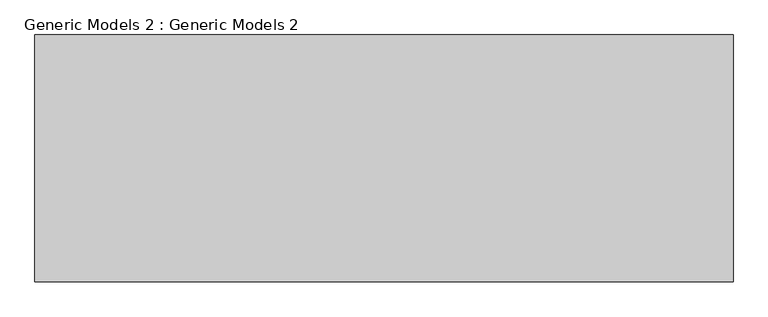
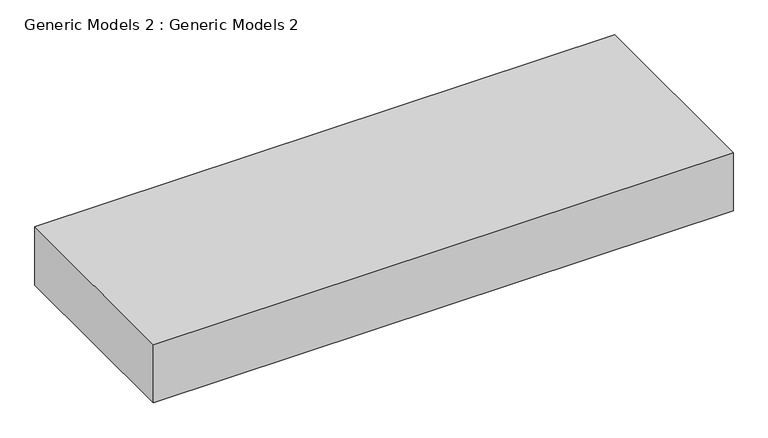
"""IFC4 building model written with IfcOpenShell, lengths in millimetres: proxy geometry, Generic Models 2 : Generic Models 2."""

from ifc_helpers import new_model, si_unit, frame, origin, place, context, project, spatial, polyline, outline, extrude, source, transform, mapped, element, save


def generic_models_2_generic_models_2_3446db89(model_context):
    return source(origin(), model_context, "Body", "SweptSolid", [
        extrude(outline(polyline([(-12143.6860997, -5429.6090801), (-15253.300702, -5429.6090801), (-15253.300702, -4329.734083), (-12143.6860997, -4329.734083), (-12143.6860997, -5429.6090801)])), frame((0.0, 0.0, 5612.8), z_axis=(0.0, 0.0, 1.0), x_axis=(1.0, 0.0, 0.0)), (0.0, 0.0, 1.0), 330.2),
    ])


if __name__ == "__main__":
    model = new_model("IFC4")
    model_context = context("Model", 3, world=origin())
    ifc_project = project(units=[si_unit("LENGTHUNIT", "METRE", prefix="MILLI")], contexts=[model_context])
    site = spatial("IfcSite", under=ifc_project)
    building = spatial("IfcBuilding", under=site)
    placement = place(None, origin())
    generic_models_2_generic_models_2_shape = generic_models_2_generic_models_2_3446db89(model_context)
    element("IfcBuildingElementProxy", 1, Name="Generic Models 2 : Generic Models 2", ObjectType="Generic Models 2 : Generic Models 2", at=placement, inside=building, context=model_context, shape_type="MappedRepresentation", body=[
        mapped(generic_models_2_generic_models_2_shape, transform((0.0, 0.0, 0.0), x_axis=(1.0, 0.0, 0.0), y_axis=(0.0, 1.0, 0.0), z_axis=(0.0, 0.0, 1.0))),
    ])
    save(model, "model.ifc")
